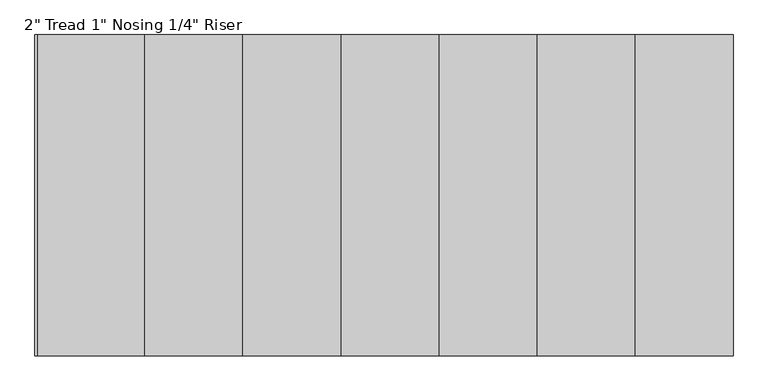
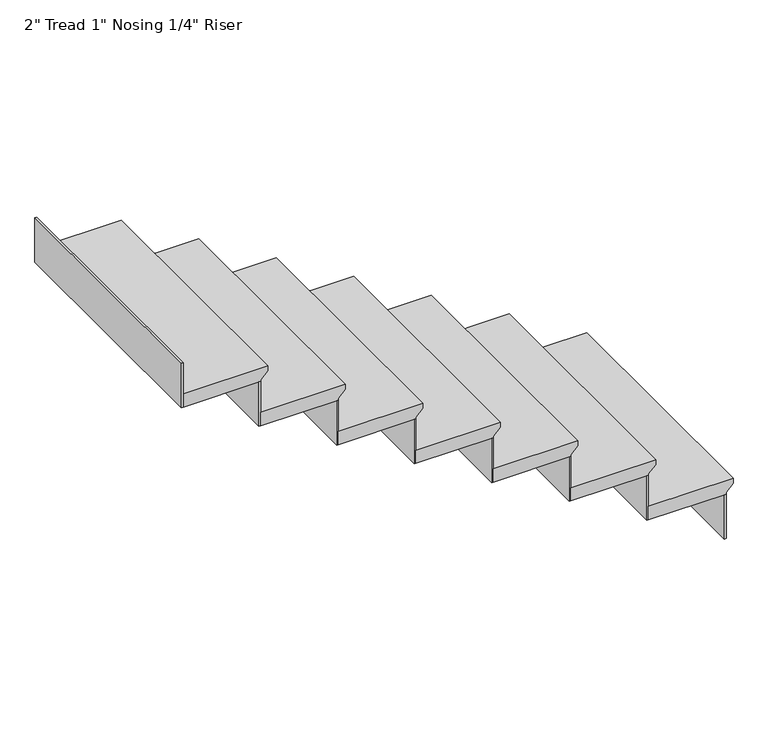
"""IFC4 building model written with IfcOpenShell, lengths in millimetres: stair flight geometry."""

from ifc_helpers import new_model, si_unit, frame, origin, place, context, project, spatial, polyline, outline, extrude, source, transform, mapped, element, save


def stair_flight_469bbda7(model_context):
    return source(origin(), model_context, "Body", "SweptSolid", [
        extrude(outline(polyline([(2032.0, -2394.7932736), (2032.0, -2699.5932736), (1981.2, -2699.5932736), (1981.2, -2420.1932736), (1987.55, -2420.1932736), (2012.95, -2394.7932736), (2032.0, -2394.7932736)])), frame((0.0, 6009.5200123, 0.0), z_axis=(0.0, 1.0, 0.0), x_axis=(0.0, 0.0, 1.0)), (0.0, 0.0, 1.0), 914.4),
        extrude(outline(polyline([(-2426.5432736, 6923.9200123), (-2420.1932736, 6923.9200123), (-2420.1932736, 6009.5200123), (-2426.5432736, 6009.5200123), (-2426.5432736, 6923.9200123)])), frame((0.0, 0.0, 1811.8666667), z_axis=(0.0, 0.0, 1.0), x_axis=(1.0, 0.0, 0.0)), (0.0, 0.0, 1.0), 169.3333333),
        extrude(outline(polyline([(-2705.9432736, 6923.9200123), (-2699.5932736, 6923.9200123), (-2699.5932736, 6009.5200123), (-2705.9432736, 6009.5200123), (-2705.9432736, 6923.9200123)])), frame((0.0, 0.0, 1981.2), z_axis=(0.0, 0.0, 1.0), x_axis=(1.0, 0.0, 0.0)), (0.0, 0.0, 1.0), 169.3333333),
        extrude(outline(polyline([(2201.3333333, -2674.1932736), (2201.3333333, -2978.9932736), (2150.5333333, -2978.9932736), (2150.5333333, -2699.5932736), (2156.8833333, -2699.5932736), (2182.2833333, -2674.1932736), (2201.3333333, -2674.1932736)])), frame((0.0, 6009.5200123, 0.0), z_axis=(0.0, 1.0, 0.0), x_axis=(0.0, 0.0, 1.0)), (0.0, 0.0, 1.0), 914.4),
        extrude(outline(polyline([(-2985.3432736, 6923.9200123), (-2978.9932736, 6923.9200123), (-2978.9932736, 6009.5200123), (-2985.3432736, 6009.5200123), (-2985.3432736, 6923.9200123)])), frame((0.0, 0.0, 2150.5333333), z_axis=(0.0, 0.0, 1.0), x_axis=(1.0, 0.0, 0.0)), (0.0, 0.0, 1.0), 169.3333333),
        extrude(outline(polyline([(2370.6666667, -2953.5932736), (2370.6666667, -3258.3932736), (2319.8666667, -3258.3932736), (2319.8666667, -2978.9932736), (2326.2166667, -2978.9932736), (2351.6166667, -2953.5932736), (2370.6666667, -2953.5932736)])), frame((0.0, 6009.5200123, 0.0), z_axis=(0.0, 1.0, 0.0), x_axis=(0.0, 0.0, 1.0)), (0.0, 0.0, 1.0), 914.4),
        extrude(outline(polyline([(-3264.7432736, 6923.9200123), (-3258.3932736, 6923.9200123), (-3258.3932736, 6009.5200123), (-3264.7432736, 6009.5200123), (-3264.7432736, 6923.9200123)])), frame((0.0, 0.0, 2319.8666667), z_axis=(0.0, 0.0, 1.0), x_axis=(1.0, 0.0, 0.0)), (0.0, 0.0, 1.0), 169.3333333),
        extrude(outline(polyline([(2540.0, -3232.9932736), (2540.0, -3537.7932736), (2489.2, -3537.7932736), (2489.2, -3258.3932736), (2495.55, -3258.3932736), (2520.95, -3232.9932736), (2540.0, -3232.9932736)])), frame((0.0, 6009.5200123, 0.0), z_axis=(0.0, 1.0, 0.0), x_axis=(0.0, 0.0, 1.0)), (0.0, 0.0, 1.0), 914.4),
        extrude(outline(polyline([(-3544.1432736, 6923.9200123), (-3537.7932736, 6923.9200123), (-3537.7932736, 6009.5200123), (-3544.1432736, 6009.5200123), (-3544.1432736, 6923.9200123)])), frame((0.0, 0.0, 2489.2), z_axis=(0.0, 0.0, 1.0), x_axis=(1.0, 0.0, 0.0)), (0.0, 0.0, 1.0), 169.3333333),
        extrude(outline(polyline([(2709.3333333, -3512.3932736), (2709.3333333, -3817.1932736), (2658.5333333, -3817.1932736), (2658.5333333, -3537.7932736), (2664.8833333, -3537.7932736), (2690.2833333, -3512.3932736), (2709.3333333, -3512.3932736)])), frame((0.0, 6009.5200123, 0.0), z_axis=(0.0, 1.0, 0.0), x_axis=(0.0, 0.0, 1.0)), (0.0, 0.0, 1.0), 914.4),
        extrude(outline(polyline([(-3823.5432736, 6923.9200123), (-3817.1932736, 6923.9200123), (-3817.1932736, 6009.5200123), (-3823.5432736, 6009.5200123), (-3823.5432736, 6923.9200123)])), frame((0.0, 0.0, 2658.5333333), z_axis=(0.0, 0.0, 1.0), x_axis=(1.0, 0.0, 0.0)), (0.0, 0.0, 1.0), 169.3333333),
        extrude(outline(polyline([(2878.6666667, -3791.7932736), (2878.6666667, -4096.5932736), (2827.8666667, -4096.5932736), (2827.8666667, -3817.1932736), (2834.2166667, -3817.1932736), (2859.6166667, -3791.7932736), (2878.6666667, -3791.7932736)])), frame((0.0, 6009.5200123, 0.0), z_axis=(0.0, 1.0, 0.0), x_axis=(0.0, 0.0, 1.0)), (0.0, 0.0, 1.0), 914.4),
        extrude(outline(polyline([(-4102.9432736, 6923.9200123), (-4096.5932736, 6923.9200123), (-4096.5932736, 6009.5200123), (-4102.9432736, 6009.5200123), (-4102.9432736, 6923.9200123)])), frame((0.0, 0.0, 2827.8666667), z_axis=(0.0, 0.0, 1.0), x_axis=(1.0, 0.0, 0.0)), (0.0, 0.0, 1.0), 169.3333333),
        extrude(outline(polyline([(-4382.3432736, 6923.9200123), (-4375.9932736, 6923.9200123), (-4375.9932736, 6009.5200123), (-4382.3432736, 6009.5200123), (-4382.3432736, 6923.9200123)])), frame((0.0, 0.0, 2997.2), z_axis=(0.0, 0.0, 1.0), x_axis=(1.0, 0.0, 0.0)), (0.0, 0.0, 1.0), 169.3333333),
        extrude(outline(polyline([(3048.0, -4071.1932736), (3048.0, -4375.9932736), (2997.2, -4375.9932736), (2997.2, -4096.5932736), (3003.55, -4096.5932736), (3028.95, -4071.1932736), (3048.0, -4071.1932736)])), frame((0.0, 6009.5200123, 0.0), z_axis=(0.0, 1.0, 0.0), x_axis=(0.0, 0.0, 1.0)), (0.0, 0.0, 1.0), 914.4),
    ])


if __name__ == "__main__":
    model = new_model("IFC4")
    model_context = context("Model", 3, world=origin())
    ifc_project = project(units=[si_unit("LENGTHUNIT", "METRE", prefix="MILLI")], contexts=[model_context])
    site = spatial("IfcSite", under=ifc_project)
    building = spatial("IfcBuilding", under=site)
    placement = place(None, origin())
    stair_flight_shape = stair_flight_469bbda7(model_context)
    element("IfcStairFlight", 1, ObjectType="2\" Tread 1\" Nosing 1/4\" Riser", at=placement, inside=building, context=model_context, shape_type="MappedRepresentation", body=[
        mapped(stair_flight_shape, transform((0.0, 0.0, 0.0), x_axis=(1.0, 0.0, 0.0), y_axis=(0.0, 1.0, 0.0), z_axis=(0.0, 0.0, 1.0))),
    ])
    save(model, "model.ifc")
